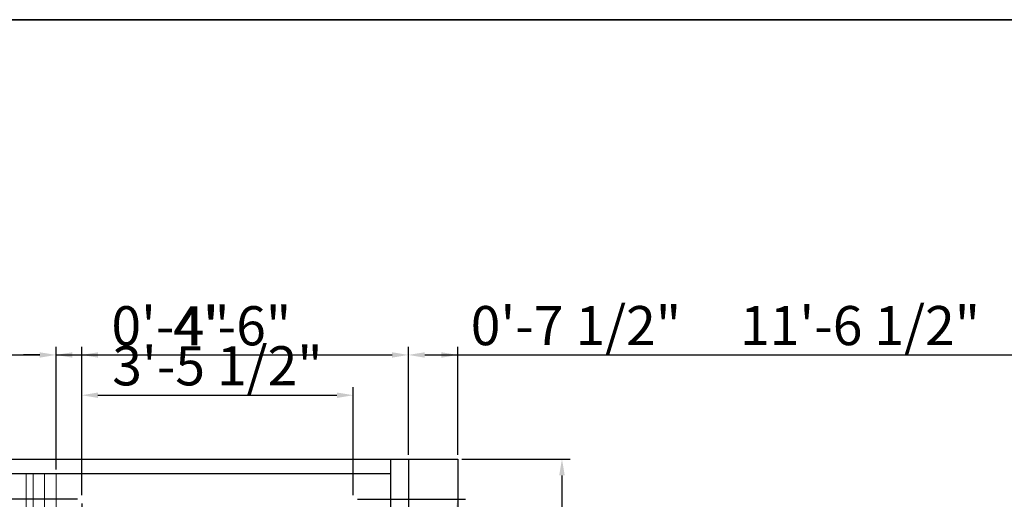
# Model space of a CAD drawing. Units: inches. Extents: x 2656 to 9931, y 1941 to 3068.
# Tile 43 of 46: x 2817 to 2968, y 2994 to 3068. Entities that reach past the tile are written whole.
import ezdxf

# ---------------------------------------------------------------- set-up
doc = ezdxf.new("R2010")
doc.units = ezdxf.units.IN
for name, color, linetype, lineweight in [('A-ANNO-DIMS', 2, 'Continuous', 18), ('A-ANNO-TTLB', 7, 'Continuous', 35), ('A-ELEV', 7, 'Continuous', 25), ('A-ELEV-FNSH', 8, 'Continuous', 13)]:
    doc.layers.add(name, color=color, linetype=linetype, lineweight=lineweight)
doc.styles.get("Standard").update_dxf_attribs({"font": 'arial.ttf'})
doc.dimstyles.new('ISO-25', dxfattribs={"dimtxt": 6, "dimasz": 2.5, "dimexe": 1.25, "dimexo": 0.625, "dimtad": 1, "dimdec": 0, "dimlunit": 3, "dimtxsty": 'Standard', "dimcen": 2.5, "dimadec": 0, "dimazin": 0, "dimtfac": 1, "dimtdec": 0, "dimtmove": 0, "dimatfit": 3, "dimfxl": 1, "dimarcsym": 0})

# ---------------------------------------------------------------- blocks, each defined once
blk = doc.blocks.new('*D83')
at = {"layer": 'A-ANNO-DIMS', "color": 0, "lineweight": -2, "transparency": 16777216}
for p, q in [((2743.16, 2998.91), (2743.16, 3017.72)), ((2822.71, 2998.91), (2822.71, 3017.72)), ((2745.66, 3016.47), (2820.21, 3016.47))]:
    blk.add_line(p, q, dxfattribs=at)
at = {"layer": 'A-ANNO-DIMS', "color": 0, "transparency": 16777216}
for points in [[(2745.66, 3016.88), (2745.66, 3016.05), (2743.16, 3016.47)], [(2820.21, 3016.88), (2820.21, 3016.05), (2822.71, 3016.47)]]:
    blk.add_solid(points, dxfattribs=at)
at = {"layer": 'Defpoints', "color": 0, "transparency": 16777216}
for p in [(2822.71, 3016.47), (2743.16, 2998.29), (2822.71, 2998.29)]:
    blk.add_point(p, dxfattribs=at)
at = {"layer": 'A-ANNO-DIMS', "color": 0, "transparency": 16777216, "insert": (2782.93, 3020.19), "char_height": 6, "attachment_point": 5}
blk.add_mtext('6\'-7 1/2"', dxfattribs=at)
blk = doc.blocks.new('*D84')
at = {"layer": 'A-ANNO-DIMS', "color": 0, "lineweight": -2, "transparency": 16777216}
for p, q in [((2822.71, 2998.91), (2822.71, 3017.72)), ((2876.66, 3001.14), (2876.66, 3017.72)), ((2825.21, 3016.47), (2874.16, 3016.47))]:
    blk.add_line(p, q, dxfattribs=at)
at = {"layer": 'A-ANNO-DIMS', "color": 0, "transparency": 16777216}
for points in [[(2825.21, 3016.88), (2825.21, 3016.05), (2822.71, 3016.47)], [(2874.16, 3016.88), (2874.16, 3016.05), (2876.66, 3016.47)]]:
    blk.add_solid(points, dxfattribs=at)
at = {"layer": 'Defpoints', "color": 0, "transparency": 16777216}
for p in [(2876.66, 3016.47), (2876.66, 3000.52), (2822.71, 2998.29)]:
    blk.add_point(p, dxfattribs=at)
at = {"layer": 'A-ANNO-DIMS', "color": 0, "transparency": 16777216, "insert": (2849.68, 3020.16), "char_height": 6, "attachment_point": 5}
blk.add_mtext('4\'-6"', dxfattribs=at)
blk = doc.blocks.new('*D85')
at = {"layer": 'A-ANNO-DIMS', "color": 0, "lineweight": -2, "transparency": 16777216}
for p, q in [((2876.66, 3001.14), (2876.66, 3017.72)), ((3014.98, 2938.52), (3014.98, 3017.72)), ((2879.16, 3016.47), (3012.48, 3016.47))]:
    blk.add_line(p, q, dxfattribs=at)
at = {"layer": 'A-ANNO-DIMS', "color": 0, "transparency": 16777216}
for points in [[(2879.16, 3016.88), (2879.16, 3016.05), (2876.66, 3016.47)], [(3012.48, 3016.88), (3012.48, 3016.05), (3014.98, 3016.47)]]:
    blk.add_solid(points, dxfattribs=at)
at = {"layer": 'Defpoints', "color": 0, "transparency": 16777216}
for p in [(3014.98, 3016.47), (2876.66, 3000.52), (3014.98, 2937.89)]:
    blk.add_point(p, dxfattribs=at)
at = {"layer": 'A-ANNO-DIMS', "color": 0, "transparency": 16777216, "insert": (2945.82, 3020.19), "char_height": 6, "attachment_point": 5}
blk.add_mtext('11\'-6 1/2"', dxfattribs=at)
blk = doc.blocks.new('*D147')
at = {"layer": 'A-ANNO-DIMS', "color": 0, "lineweight": -2, "transparency": 16777216}
for p, q in [((2822.71, 2998.91), (2822.71, 3017.72)), ((2826.64, 2994.97), (2826.64, 3017.72)), ((2820.21, 3016.47), (2817.71, 3016.47)), ((2822.71, 3016.47), (2826.64, 3016.47)), ((2829.14, 3016.47), (2848.84, 3016.47))]:
    blk.add_line(p, q, dxfattribs=at)
at = {"layer": 'A-ANNO-DIMS', "color": 0, "transparency": 16777216}
for points in [[(2820.21, 3016.88), (2820.21, 3016.05), (2822.71, 3016.47)], [(2829.14, 3016.88), (2829.14, 3016.05), (2826.64, 3016.47)]]:
    blk.add_solid(points, dxfattribs=at)
at = {"layer": 'Defpoints', "color": 0, "transparency": 16777216}
for p in [(2826.64, 3016.47), (2822.71, 2998.29), (2826.64, 2994.35)]:
    blk.add_point(p, dxfattribs=at)
at = {"layer": 'A-ANNO-DIMS', "color": 0, "transparency": 16777216, "insert": (2840.24, 3020.16), "char_height": 6, "attachment_point": 5}
blk.add_mtext('0\'-4"', dxfattribs=at)
blk = doc.blocks.new('*D148')
at = {"layer": 'A-ANNO-DIMS', "color": 0, "lineweight": -2, "transparency": 16777216}
for p, q in [((2826.64, 2994.97), (2826.64, 3011.55)), ((2868.23, 2994.97), (2868.23, 3011.55)), ((2829.14, 3010.3), (2865.73, 3010.3))]:
    blk.add_line(p, q, dxfattribs=at)
at = {"layer": 'A-ANNO-DIMS', "color": 0, "transparency": 16777216}
for points in [[(2829.14, 3010.71), (2829.14, 3009.88), (2826.64, 3010.3)], [(2865.73, 3010.71), (2865.73, 3009.88), (2868.23, 3010.3)]]:
    blk.add_solid(points, dxfattribs=at)
at = {"layer": 'Defpoints', "color": 0, "transparency": 16777216}
for p in [(2868.23, 3010.3), (2826.64, 2994.35), (2868.23, 2994.35)]:
    blk.add_point(p, dxfattribs=at)
at = {"layer": 'A-ANNO-DIMS', "color": 0, "transparency": 16777216, "insert": (2847.43, 3014.03), "char_height": 6, "attachment_point": 5}
blk.add_mtext('3\'-5 1/2"', dxfattribs=at)
blk = doc.blocks.new('*D149')
at = {"layer": 'A-ANNO-DIMS', "color": 0, "lineweight": -2, "transparency": 16777216}
for p, q in [((2868.85, 2994.35), (2885.43, 2994.35)), ((2884.18, 2991.85), (2884.18, 2894.54)), ((2868.85, 2892.04), (2885.43, 2892.04))]:
    blk.add_line(p, q, dxfattribs=at)
at = {"layer": 'A-ANNO-DIMS', "color": 0, "transparency": 16777216}
for points in [[(2883.76, 2991.85), (2884.59, 2991.85), (2884.18, 2994.35)], [(2883.76, 2894.54), (2884.59, 2894.54), (2884.18, 2892.04)]]:
    blk.add_solid(points, dxfattribs=at)
at = {"layer": 'Defpoints', "color": 0, "transparency": 16777216}
for p in [(2868.23, 2994.35), (2868.23, 2892.04), (2884.18, 2892.04)]:
    blk.add_point(p, dxfattribs=at)
at = {"layer": 'A-ANNO-DIMS', "color": 0, "transparency": 16777216, "insert": (2880.45, 2943.19), "char_height": 6, "attachment_point": 5, "rotation": 90}
blk.add_mtext('8\'-6 1/2"', dxfattribs=at)
blk = doc.blocks.new('*D153')
at = {"layer": 'A-ANNO-DIMS', "color": 0, "lineweight": -2, "transparency": 16777216}
for p, q in [((2826.64, 2993.72), (2826.64, 2703.71)), ((2829.55, 2956.42), (2829.55, 2703.71)), ((2824.14, 2704.96), (2821.64, 2704.96)), ((2826.64, 2704.96), (2829.55, 2704.96)), ((2832.05, 2704.96), (2851.75, 2704.96))]:
    blk.add_line(p, q, dxfattribs=at)
at = {"layer": 'A-ANNO-DIMS', "color": 0, "transparency": 16777216}
for points in [[(2824.14, 2705.38), (2824.14, 2704.54), (2826.64, 2704.96)], [(2832.05, 2705.38), (2832.05, 2704.54), (2829.55, 2704.96)]]:
    blk.add_solid(points, dxfattribs=at)
at = {"layer": 'Defpoints', "color": 0, "transparency": 16777216}
for p in [(2826.64, 2994.35), (2829.55, 2957.05), (2829.55, 2704.96)]:
    blk.add_point(p, dxfattribs=at)
at = {"layer": 'A-ANNO-DIMS', "color": 0, "transparency": 16777216, "insert": (2843.15, 2708.65), "char_height": 6, "attachment_point": 5}
blk.add_mtext('0\'-3"', dxfattribs=at)
blk = doc.blocks.new('*D154')
at = {"layer": 'A-ANNO-DIMS', "color": 0, "lineweight": -2, "transparency": 16777216}
for p, q in [((2708.57, 2996.85), (2708.57, 2999.35)), ((2826.02, 2994.35), (2707.32, 2994.35)), ((2708.57, 2994.35), (2708.57, 2990.83)), ((2847.28, 2990.83), (2707.32, 2990.83)), ((2708.57, 2988.33), (2708.57, 2954.65))]:
    blk.add_line(p, q, dxfattribs=at)
at = {"layer": 'A-ANNO-DIMS', "color": 0, "transparency": 16777216}
for points in [[(2708.16, 2996.85), (2708.99, 2996.85), (2708.57, 2994.35)], [(2708.16, 2988.33), (2708.99, 2988.33), (2708.57, 2990.83)]]:
    blk.add_solid(points, dxfattribs=at)
at = {"layer": 'Defpoints', "color": 0, "transparency": 16777216}
for p in [(2826.64, 2994.35), (2708.57, 2990.83), (2847.9, 2990.83)]:
    blk.add_point(p, dxfattribs=at)
at = {"layer": 'A-ANNO-DIMS', "color": 0, "transparency": 16777216, "insert": (2704.84, 2970.24), "char_height": 6, "attachment_point": 5, "rotation": 90}
blk.add_mtext('0\'-3 1/2"', dxfattribs=at)
blk = doc.blocks.new('*D164')
at = {"layer": 'A-ANNO-DIMS', "color": 0, "lineweight": -2, "transparency": 16777216}
for p, q in [((2876.66, 3001.14), (2876.66, 3017.72)), ((2884.23, 3001.14), (2884.23, 3017.72)), ((2879.16, 3016.47), (2881.73, 3016.47)), ((2884.23, 3016.47), (2917.91, 3016.47))]:
    blk.add_line(p, q, dxfattribs=at)
at = {"layer": 'A-ANNO-DIMS', "color": 0, "transparency": 16777216}
for points in [[(2879.16, 3016.88), (2879.16, 3016.05), (2876.66, 3016.47)], [(2881.73, 3016.88), (2881.73, 3016.05), (2884.23, 3016.47)]]:
    blk.add_solid(points, dxfattribs=at)
at = {"layer": 'Defpoints', "color": 0, "transparency": 16777216}
for p in [(2884.23, 3016.47), (2876.66, 3000.52), (2884.23, 3000.52)]:
    blk.add_point(p, dxfattribs=at)
at = {"layer": 'A-ANNO-DIMS', "color": 0, "transparency": 16777216, "insert": (2902.32, 3020.19), "char_height": 6, "attachment_point": 5}
blk.add_mtext('0\'-7 1/2"', dxfattribs=at)
blk = doc.blocks.new('*D165')
at = {"layer": 'A-ANNO-DIMS', "color": 0, "lineweight": -2, "transparency": 16777216}
for p, q in [((2884.85, 3000.52), (2901.43, 3000.52)), ((2900.18, 2998.02), (2900.18, 2993.16)), ((2884.85, 2990.66), (2901.43, 2990.66)), ((2900.18, 2990.66), (2900.18, 2966.3))]:
    blk.add_line(p, q, dxfattribs=at)
at = {"layer": 'A-ANNO-DIMS', "color": 0, "transparency": 16777216}
for points in [[(2899.76, 2998.02), (2900.6, 2998.02), (2900.18, 3000.52)], [(2899.76, 2993.16), (2900.6, 2993.16), (2900.18, 2990.66)]]:
    blk.add_solid(points, dxfattribs=at)
at = {"layer": 'Defpoints', "color": 0, "transparency": 16777216}
for p in [(2884.23, 3000.52), (2884.23, 2990.66), (2900.18, 2990.66)]:
    blk.add_point(p, dxfattribs=at)
at = {"layer": 'A-ANNO-DIMS', "color": 0, "transparency": 16777216, "insert": (2896.49, 2977.23), "char_height": 6, "attachment_point": 5, "rotation": 90}
blk.add_mtext('0\'-10"', dxfattribs=at)

msp = doc.modelspace()

# ---------------------------------------------------------------- linework, layer by layer
at = {"layer": 'A-ANNO-TTLB'}
msp.add_lwpolyline([(2655.77, 3067.84), (3515.43, 3067.84), (3515.43, 1940.89), (2655.77, 1940.89)], close=True, dxfattribs=at)
at = {"layer": 'A-ELEV'}
for p, q in [((2743.16, 3000.52), (2884.23, 3000.52)), ((2876.66, 3000.52), (2876.66, 2935.89)), ((2884.23, 3000.52), (2884.23, 2990.66)), ((2746.62, 2998.29), (2873.91, 2998.29))]:
    msp.add_line(p, q, dxfattribs=at)
msp.add_lwpolyline([(2873.91, 3000.52), (2873.91, 2898.94)], dxfattribs=at)
at = {"layer": 'A-ELEV-FNSH'}
for p, q in [((2818.13, 2887.89), (2818.13, 2998.29)), ((2819.23, 2887.89), (2819.23, 2998.29)), ((2820.95, 2887.89), (2820.95, 2998.29)), ((2822.71, 2887.89), (2822.71, 2998.29))]:
    msp.add_line(p, q, dxfattribs=at)

# ---------------------------------------------------------------- dimensions: what is measured, and where the dimension line sits
at = {"layer": 'A-ANNO-DIMS'}
for base, p1, p2, picture, middle in [((2822.7053, 3016.4671), (2743.1573, 2998.2859), (2822.7053, 2998.2859), '*D83', (2782.9313, 3020.1944)), ((3014.98, 3016.47), (2876.66, 3000.52), (3014.98, 2937.89), '*D85', (2945.82, 3020.19)), ((2884.23, 3016.47), (2876.66, 3000.52), (2884.23, 3000.52), '*D164', (2902.32, 3020.19)), ((2826.64, 3016.47), (2822.71, 2998.29), (2826.64, 2994.35), '*D147', (2840.24, 3020.16)), ((2876.6573, 3016.4671), (2822.7053, 2998.2859), (2876.6573, 3000.5171), '*D84', (2849.6813, 3020.1555)), ((2868.23, 3010.3), (2826.64, 2994.35), (2868.23, 2994.35), '*D148', (2847.43, 3014.03)), ((2829.55, 2704.96), (2826.64, 2994.35), (2829.55, 2957.05), '*D153', (2843.15, 2708.65))]:
    dim = msp.add_linear_dim(base=base, p1=p1, p2=p2, dimstyle='ISO-25', override={"dimdec": 1, "dimlfac": 1, "dimrnd": 0, "dimzin": 1, "dimdsep": 46, "dimlunit": 4, "dimfrac": 2}, dxfattribs=at)
    dim.commit()
    dim.dimension.update_dxf_attribs({"geometry": picture, "text_midpoint": middle})
for base, p1, p2, angle, picture, middle in [((2900.18, 2990.66), (2884.23, 3000.52), (2884.23, 2990.66), 270, '*D165', (2896.49, 2977.23)), ((2708.57, 2990.83), (2826.64, 2994.35), (2847.9, 2990.83), 90, '*D154', (2704.84, 2970.24)), ((2884.18, 2892.04), (2868.23, 2994.35), (2868.23, 2892.04), 270, '*D149', (2880.45, 2943.19))]:
    dim = msp.add_linear_dim(base=base, p1=p1, p2=p2, angle=angle, dimstyle='ISO-25', override={"dimdec": 1, "dimlfac": 1, "dimrnd": 0, "dimzin": 1, "dimdsep": 46, "dimlunit": 4, "dimfrac": 2}, dxfattribs=at)
    dim.commit()
    dim.dimension.update_dxf_attribs({"geometry": picture, "text_midpoint": middle})

doc.saveas('drawing.dxf')
